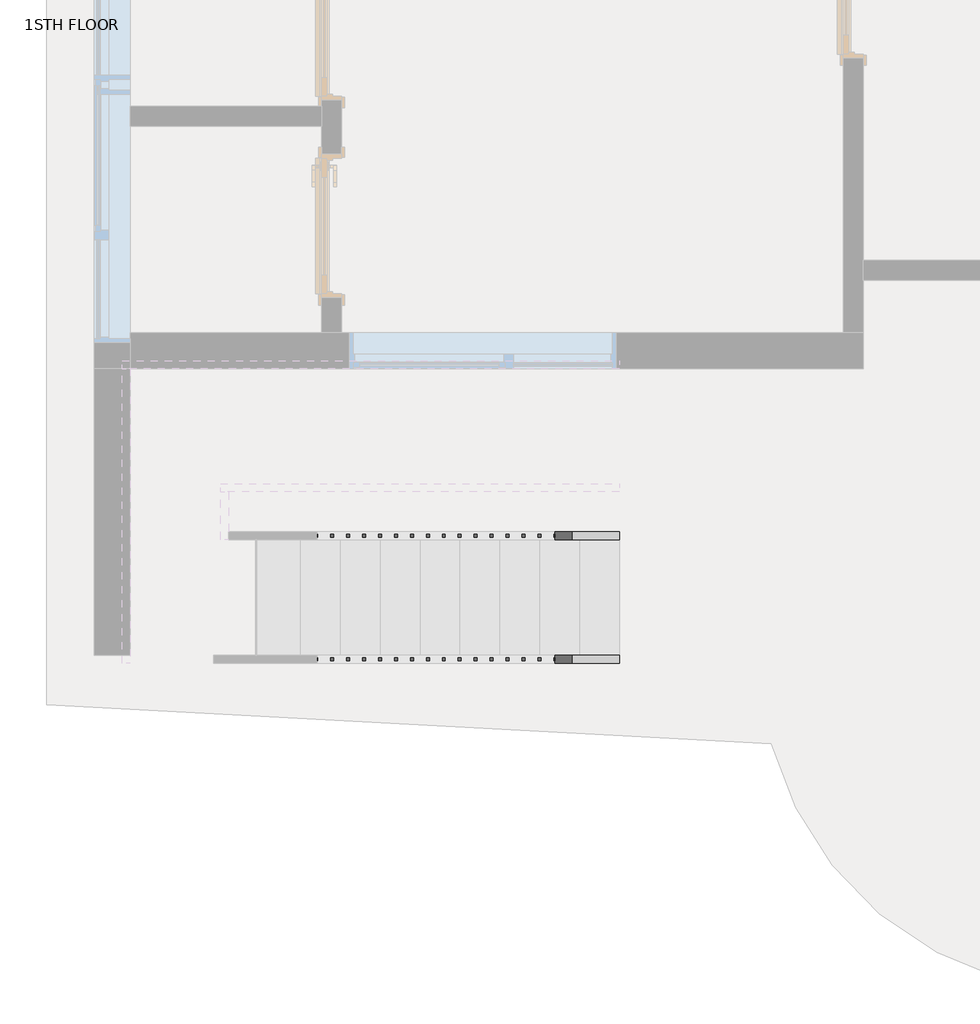
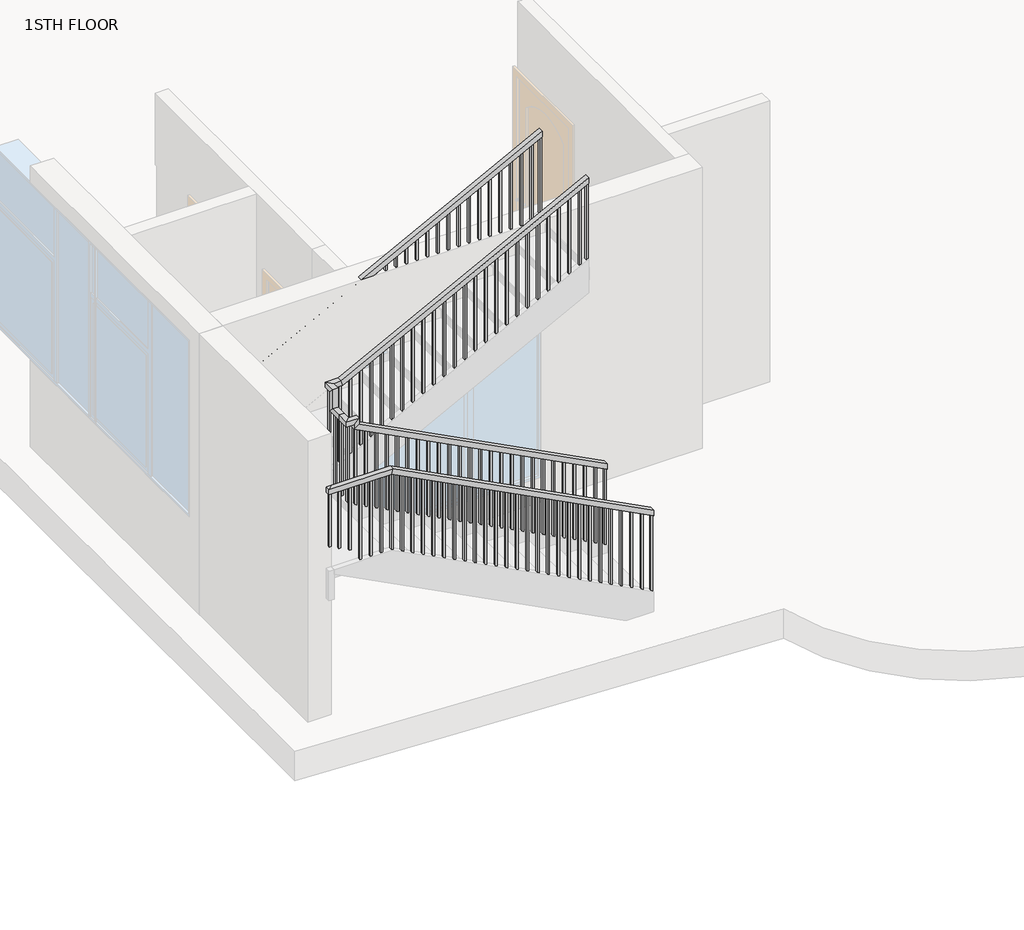
# One storey, part 3 of 4: 2 railings.
"""IFC4 building model written with IfcOpenShell, lengths in millimetres."""

from ifc_helpers import new_model, si_unit, frame, origin, place, context, project, spatial, polyline, outline, extrude, faceted_brep, element, save

model = new_model("IFC4")

# Units and contexts
model_context = context("Model", 3, world=origin())
ifc_project = project(units=[si_unit("LENGTHUNIT", "METRE", prefix="MILLI")], contexts=[model_context])

# Site, building, storey
site = spatial("IfcSite", under=ifc_project)
building = spatial("IfcBuilding", under=site)
storey = spatial("IfcBuildingStorey", under=building, Name="1STH FLOOR", Elevation=3200.4)

# Railings
placement = place(None, origin())
element("IfcRailing", 1, ObjectType="Handrail - Rectangular", at=placement, inside=storey, context=model_context, shape_type="SolidModel", body=[
    faceted_brep([(-3117.2664982, -6914.3822004, 4246.4181818), (-3117.2664982, -6914.3822004, 4189.203028), (-3117.2664982, -6863.5822004, 4189.203028), (-3117.2664982, -6863.5822004, 4246.4181818), (-5530.2664982, -6914.3822004, 5496.7909091), (-5581.0664982, -6914.3822004, 5465.8993916), (-5581.0664982, -6863.5822004, 5465.8993916), (-5530.2664982, -6863.5822004, 5496.7909091), (-5657.2664982, -6787.3822004, 5511.8), (-5657.2664982, -6787.3822004, 5562.6), (-5657.2664982, -6685.7822004, 5562.6), (-5657.2664982, -6634.9822004, 5511.8), (-5606.4664982, -6787.3822004, 5511.8), (-5606.4664982, -6634.9822004, 5511.8), (-5606.4664982, -6787.3822004, 5562.6), (-5606.4664982, -6685.7822004, 5562.6), (-3117.2664982, -6558.7822004, 7010.4), (-3117.2664982, -6609.5822004, 7010.4), (-3117.2664982, -6609.5822004, 6953.1848461), (-3117.2664982, -6558.7822004, 6953.1848461), (-5517.8863767, -6558.7822004, 5709.2272727), (-5530.2664982, -6558.7822004, 5760.0272727), (-5517.8863767, -6609.5822004, 5709.2272727), (-5530.2664982, -6609.5822004, 5760.0272727), (-5530.2664982, -6914.3822004, 5562.6), (-5581.0664982, -6914.3822004, 5511.8), (-5581.0664982, -6863.5822004, 5511.8), (-5530.2664982, -6863.5822004, 5562.6), (-5657.2664982, -6914.3822004, 5562.6), (-5657.2664982, -6914.3822004, 5511.8), (-5606.4664982, -6863.5822004, 5511.8), (-5606.4664982, -6863.5822004, 5562.6), (-5657.2664982, -6685.7822004, 5760.0272727), (-5657.2664982, -6634.9822004, 5709.2272727), (-5606.4664982, -6634.9822004, 5709.2272727), (-5606.4664982, -6685.7822004, 5760.0272727), (-5657.2664982, -6558.7822004, 5760.0272727), (-5657.2664982, -6558.7822004, 5709.2272727), (-5606.4664982, -6609.5822004, 5709.2272727), (-5606.4664982, -6609.5822004, 5760.0272727)], [[[0, 1, 2, 3]], [[1, 0, 4, 5]], [[2, 1, 5, 6]], [[3, 2, 6, 7]], [[0, 3, 7, 4]], [[8, 9, 10, 11]], [[12, 8, 11, 13]], [[14, 12, 13, 15]], [[9, 14, 15, 10]], [[16, 17, 18, 19]], [[20, 21, 16, 19]], [[22, 20, 19, 18]], [[23, 22, 18, 17]], [[21, 23, 17, 16]], [[5, 4, 24, 25]], [[6, 5, 25, 26]], [[7, 6, 26, 27]], [[4, 7, 27, 24]], [[25, 24, 28, 29]], [[26, 25, 29, 30]], [[27, 26, 30, 31]], [[24, 27, 31, 28]], [[29, 28, 9, 8]], [[30, 29, 8, 12]], [[31, 30, 12, 14]], [[28, 31, 14, 9]], [[11, 10, 32, 33]], [[13, 11, 33, 34]], [[15, 13, 34, 35]], [[10, 15, 35, 32]], [[33, 32, 36, 37]], [[34, 33, 37, 38]], [[35, 34, 38, 39]], [[32, 35, 39, 36]], [[37, 36, 21, 20]], [[38, 37, 20, 22]], [[39, 38, 22, 23]], [[36, 39, 23, 21]]]),
    extrude(outline(polyline([(6918.6350734, -3183.9414982), (6908.7637098, -3202.9914982), (6124.4803899, -3202.9914982), (6134.3517536, -3183.9414982), (6918.6350734, -3183.9414982)])), frame((0.0, -6593.7072004, 0.0), z_axis=(0.0, 1.0, 0.0), x_axis=(0.0, 0.0, 1.0)), (0.0, 0.0, 1.0), 19.05),
    extrude(outline(polyline([(6865.9878007, -3285.5414982), (6856.116437, -3304.5914982), (6071.8331172, -3304.5914982), (6081.7044808, -3285.5414982), (6865.9878007, -3285.5414982)])), frame((0.0, -6593.7072004, 0.0), z_axis=(0.0, 1.0, 0.0), x_axis=(0.0, 0.0, 1.0)), (0.0, 0.0, 1.0), 19.05),
    extrude(outline(polyline([(6813.340528, -3387.1414982), (6803.4691643, -3406.1914982), (6019.1858445, -3406.1914982), (6029.0572081, -3387.1414982), (6813.340528, -3387.1414982)])), frame((0.0, -6593.7072004, 0.0), z_axis=(0.0, 1.0, 0.0), x_axis=(0.0, 0.0, 1.0)), (0.0, 0.0, 1.0), 19.05),
    extrude(outline(polyline([(6760.6932552, -3488.7414982), (6750.8218916, -3507.7914982), (5966.5385718, -3507.7914982), (5976.4099354, -3488.7414982), (6760.6932552, -3488.7414982)])), frame((0.0, -6593.7072004, 0.0), z_axis=(0.0, 1.0, 0.0), x_axis=(0.0, 0.0, 1.0)), (0.0, 0.0, 1.0), 19.05),
    extrude(outline(polyline([(6708.0459825, -3590.3414982), (6698.1746189, -3609.3914982), (5913.891299, -3609.3914982), (5923.7626627, -3590.3414982), (6708.0459825, -3590.3414982)])), frame((0.0, -6593.7072004, 0.0), z_axis=(0.0, 1.0, 0.0), x_axis=(0.0, 0.0, 1.0)), (0.0, 0.0, 1.0), 19.05),
    extrude(outline(polyline([(6655.3987098, -3691.9414982), (6645.5273461, -3710.9914982), (5861.2440263, -3710.9914982), (5871.1153899, -3691.9414982), (6655.3987098, -3691.9414982)])), frame((0.0, -6593.7072004, 0.0), z_axis=(0.0, 1.0, 0.0), x_axis=(0.0, 0.0, 1.0)), (0.0, 0.0, 1.0), 19.05),
    extrude(outline(polyline([(6602.751437, -3793.5414982), (6592.8800734, -3812.5914982), (5808.5967536, -3812.5914982), (5818.4681172, -3793.5414982), (6602.751437, -3793.5414982)])), frame((0.0, -6593.7072004, 0.0), z_axis=(0.0, 1.0, 0.0), x_axis=(0.0, 0.0, 1.0)), (0.0, 0.0, 1.0), 19.05),
    extrude(outline(polyline([(6550.1041643, -3895.1414982), (6540.2328007, -3914.1914982), (5755.9494808, -3914.1914982), (5765.8208445, -3895.1414982), (6550.1041643, -3895.1414982)])), frame((0.0, -6593.7072004, 0.0), z_axis=(0.0, 1.0, 0.0), x_axis=(0.0, 0.0, 1.0)), (0.0, 0.0, 1.0), 19.05),
    extrude(outline(polyline([(6497.4568916, -3996.7414982), (6487.585528, -4015.7914982), (5703.3022081, -4015.7914982), (5713.1735718, -3996.7414982), (6497.4568916, -3996.7414982)])), frame((0.0, -6593.7072004, 0.0), z_axis=(0.0, 1.0, 0.0), x_axis=(0.0, 0.0, 1.0)), (0.0, 0.0, 1.0), 19.05),
    extrude(outline(polyline([(6444.8096189, -4098.3414982), (6434.9382552, -4117.3914982), (5650.6549354, -4117.3914982), (5660.526299, -4098.3414982), (6444.8096189, -4098.3414982)])), frame((0.0, -6593.7072004, 0.0), z_axis=(0.0, 1.0, 0.0), x_axis=(0.0, 0.0, 1.0)), (0.0, 0.0, 1.0), 19.05),
    extrude(outline(polyline([(6392.1623461, -4199.9414982), (6382.2909825, -4218.9914982), (5598.0076627, -4218.9914982), (5607.8790263, -4199.9414982), (6392.1623461, -4199.9414982)])), frame((0.0, -6593.7072004, 0.0), z_axis=(0.0, 1.0, 0.0), x_axis=(0.0, 0.0, 1.0)), (0.0, 0.0, 1.0), 19.05),
    extrude(outline(polyline([(6339.5150734, -4301.5414982), (6329.6437098, -4320.5914982), (5545.3603899, -4320.5914982), (5555.2317536, -4301.5414982), (6339.5150734, -4301.5414982)])), frame((0.0, -6593.7072004, 0.0), z_axis=(0.0, 1.0, 0.0), x_axis=(0.0, 0.0, 1.0)), (0.0, 0.0, 1.0), 19.05),
    extrude(outline(polyline([(6286.8678007, -4403.1414982), (6276.996437, -4422.1914982), (5492.7131172, -4422.1914982), (5502.5844808, -4403.1414982), (6286.8678007, -4403.1414982)])), frame((0.0, -6593.7072004, 0.0), z_axis=(0.0, 1.0, 0.0), x_axis=(0.0, 0.0, 1.0)), (0.0, 0.0, 1.0), 19.05),
    extrude(outline(polyline([(6234.220528, -4504.7414982), (6224.3491643, -4523.7914982), (5440.0658445, -4523.7914982), (5449.9372081, -4504.7414982), (6234.220528, -4504.7414982)])), frame((0.0, -6593.7072004, 0.0), z_axis=(0.0, 1.0, 0.0), x_axis=(0.0, 0.0, 1.0)), (0.0, 0.0, 1.0), 19.05),
    extrude(outline(polyline([(6181.5732552, -4606.3414982), (6171.7018916, -4625.3914982), (5387.4185718, -4625.3914982), (5397.2899354, -4606.3414982), (6181.5732552, -4606.3414982)])), frame((0.0, -6593.7072004, 0.0), z_axis=(0.0, 1.0, 0.0), x_axis=(0.0, 0.0, 1.0)), (0.0, 0.0, 1.0), 19.05),
    extrude(outline(polyline([(6128.9259825, -4707.9414982), (6119.0546189, -4726.9914982), (5334.771299, -4726.9914982), (5344.6426627, -4707.9414982), (6128.9259825, -4707.9414982)])), frame((0.0, -6593.7072004, 0.0), z_axis=(0.0, 1.0, 0.0), x_axis=(0.0, 0.0, 1.0)), (0.0, 0.0, 1.0), 19.05),
    extrude(outline(polyline([(6076.2787098, -4809.5414982), (6066.4073461, -4828.5914982), (5282.1240263, -4828.5914982), (5291.9953899, -4809.5414982), (6076.2787098, -4809.5414982)])), frame((0.0, -6593.7072004, 0.0), z_axis=(0.0, 1.0, 0.0), x_axis=(0.0, 0.0, 1.0)), (0.0, 0.0, 1.0), 19.05),
    extrude(outline(polyline([(6023.631437, -4911.1414982), (6013.7600734, -4930.1914982), (5229.4767536, -4930.1914982), (5239.3481172, -4911.1414982), (6023.631437, -4911.1414982)])), frame((0.0, -6593.7072004, 0.0), z_axis=(0.0, 1.0, 0.0), x_axis=(0.0, 0.0, 1.0)), (0.0, 0.0, 1.0), 19.05),
    extrude(outline(polyline([(5970.9841643, -5012.7414982), (5961.1128007, -5031.7914982), (5176.8294808, -5031.7914982), (5186.7008445, -5012.7414982), (5970.9841643, -5012.7414982)])), frame((0.0, -6593.7072004, 0.0), z_axis=(0.0, 1.0, 0.0), x_axis=(0.0, 0.0, 1.0)), (0.0, 0.0, 1.0), 19.05),
    extrude(outline(polyline([(5918.3368916, -5114.3414982), (5908.465528, -5133.3914982), (5124.1822081, -5133.3914982), (5134.0535718, -5114.3414982), (5918.3368916, -5114.3414982)])), frame((0.0, -6593.7072004, 0.0), z_axis=(0.0, 1.0, 0.0), x_axis=(0.0, 0.0, 1.0)), (0.0, 0.0, 1.0), 19.05),
    extrude(outline(polyline([(5865.6896189, -5215.9414982), (5855.8182552, -5234.9914982), (5071.5349354, -5234.9914982), (5081.406299, -5215.9414982), (5865.6896189, -5215.9414982)])), frame((0.0, -6593.7072004, 0.0), z_axis=(0.0, 1.0, 0.0), x_axis=(0.0, 0.0, 1.0)), (0.0, 0.0, 1.0), 19.05),
    extrude(outline(polyline([(5813.0423461, -5317.5414982), (5803.1709825, -5336.5914982), (5018.8876627, -5336.5914982), (5028.7590263, -5317.5414982), (5813.0423461, -5317.5414982)])), frame((0.0, -6593.7072004, 0.0), z_axis=(0.0, 1.0, 0.0), x_axis=(0.0, 0.0, 1.0)), (0.0, 0.0, 1.0), 19.05),
    extrude(outline(polyline([(5760.3950734, -5419.1414982), (5750.5237098, -5438.1914982), (4966.2403899, -5438.1914982), (4976.1117536, -5419.1414982), (5760.3950734, -5419.1414982)])), frame((0.0, -6593.7072004, 0.0), z_axis=(0.0, 1.0, 0.0), x_axis=(0.0, 0.0, 1.0)), (0.0, 0.0, 1.0), 19.05),
    extrude(outline(polyline([(5707.7478007, -5520.7414982), (5697.876437, -5539.7914982), (4913.5931172, -5539.7914982), (4923.4644808, -5520.7414982), (5707.7478007, -5520.7414982)])), frame((0.0, -6593.7072004, 0.0), z_axis=(0.0, 1.0, 0.0), x_axis=(0.0, 0.0, 1.0)), (0.0, 0.0, 1.0), 19.05),
    extrude(outline(polyline([(-5622.3414982, -6695.3072004), (-5641.3914982, -6695.3072004), (-5641.3914982, -6676.2572004), (-5622.3414982, -6676.2572004), (-5622.3414982, -6695.3072004)])), frame((0.0, 0.0, 4724.4), z_axis=(0.0, 0.0, 1.0), x_axis=(1.0, 0.0, 0.0)), (0.0, 0.0, 1.0), 787.4),
    extrude(outline(polyline([(-5622.3414982, -6796.9072004), (-5641.3914982, -6796.9072004), (-5641.3914982, -6777.8572004), (-5622.3414982, -6777.8572004), (-5622.3414982, -6796.9072004)])), frame((0.0, 0.0, 4724.4), z_axis=(0.0, 0.0, 1.0), x_axis=(1.0, 0.0, 0.0)), (0.0, 0.0, 1.0), 787.4),
    extrude(outline(polyline([(5511.8, -5546.1414982), (5511.8, -5565.1914982), (4673.3899354, -5565.1914982), (4663.5185718, -5546.1414982), (5511.8, -5546.1414982)])), frame((0.0, -6898.5072004, 0.0), z_axis=(0.0, 1.0, 0.0), x_axis=(0.0, 0.0, 1.0)), (0.0, 0.0, 1.0), 19.05),
    extrude(outline(polyline([(5395.1546189, -5444.5414982), (5405.0259825, -5463.5914982), (4620.7426627, -5463.5914982), (4610.871299, -5444.5414982), (5395.1546189, -5444.5414982)])), frame((0.0, -6898.5072004, 0.0), z_axis=(0.0, 1.0, 0.0), x_axis=(0.0, 0.0, 1.0)), (0.0, 0.0, 1.0), 19.05),
    extrude(outline(polyline([(5342.5073461, -5342.9414982), (5352.3787098, -5361.9914982), (4568.0953899, -5361.9914982), (4558.2240263, -5342.9414982), (5342.5073461, -5342.9414982)])), frame((0.0, -6898.5072004, 0.0), z_axis=(0.0, 1.0, 0.0), x_axis=(0.0, 0.0, 1.0)), (0.0, 0.0, 1.0), 19.05),
    extrude(outline(polyline([(5289.8600734, -5241.3414982), (5299.731437, -5260.3914982), (4515.4481172, -5260.3914982), (4505.5767536, -5241.3414982), (5289.8600734, -5241.3414982)])), frame((0.0, -6898.5072004, 0.0), z_axis=(0.0, 1.0, 0.0), x_axis=(0.0, 0.0, 1.0)), (0.0, 0.0, 1.0), 19.05),
    extrude(outline(polyline([(5237.2128007, -5139.7414982), (5247.0841643, -5158.7914982), (4462.8008445, -5158.7914982), (4452.9294808, -5139.7414982), (5237.2128007, -5139.7414982)])), frame((0.0, -6898.5072004, 0.0), z_axis=(0.0, 1.0, 0.0), x_axis=(0.0, 0.0, 1.0)), (0.0, 0.0, 1.0), 19.05),
    extrude(outline(polyline([(5184.565528, -5038.1414982), (5194.4368916, -5057.1914982), (4410.1535718, -5057.1914982), (4400.2822081, -5038.1414982), (5184.565528, -5038.1414982)])), frame((0.0, -6898.5072004, 0.0), z_axis=(0.0, 1.0, 0.0), x_axis=(0.0, 0.0, 1.0)), (0.0, 0.0, 1.0), 19.05),
    extrude(outline(polyline([(5131.9182552, -4936.5414982), (5141.7896189, -4955.5914982), (4357.506299, -4955.5914982), (4347.6349354, -4936.5414982), (5131.9182552, -4936.5414982)])), frame((0.0, -6898.5072004, 0.0), z_axis=(0.0, 1.0, 0.0), x_axis=(0.0, 0.0, 1.0)), (0.0, 0.0, 1.0), 19.05),
    extrude(outline(polyline([(5079.2709825, -4834.9414982), (5089.1423461, -4853.9914982), (4304.8590263, -4853.9914982), (4294.9876627, -4834.9414982), (5079.2709825, -4834.9414982)])), frame((0.0, -6898.5072004, 0.0), z_axis=(0.0, 1.0, 0.0), x_axis=(0.0, 0.0, 1.0)), (0.0, 0.0, 1.0), 19.05),
    extrude(outline(polyline([(5026.6237098, -4733.3414982), (5036.4950734, -4752.3914982), (4252.2117536, -4752.3914982), (4242.3403899, -4733.3414982), (5026.6237098, -4733.3414982)])), frame((0.0, -6898.5072004, 0.0), z_axis=(0.0, 1.0, 0.0), x_axis=(0.0, 0.0, 1.0)), (0.0, 0.0, 1.0), 19.05),
    extrude(outline(polyline([(4973.976437, -4631.7414982), (4983.8478007, -4650.7914982), (4199.5644808, -4650.7914982), (4189.6931172, -4631.7414982), (4973.976437, -4631.7414982)])), frame((0.0, -6898.5072004, 0.0), z_axis=(0.0, 1.0, 0.0), x_axis=(0.0, 0.0, 1.0)), (0.0, 0.0, 1.0), 19.05),
    extrude(outline(polyline([(4921.3291643, -4530.1414982), (4931.200528, -4549.1914982), (4146.9172081, -4549.1914982), (4137.0458445, -4530.1414982), (4921.3291643, -4530.1414982)])), frame((0.0, -6898.5072004, 0.0), z_axis=(0.0, 1.0, 0.0), x_axis=(0.0, 0.0, 1.0)), (0.0, 0.0, 1.0), 19.05),
    extrude(outline(polyline([(4868.6818916, -4428.5414982), (4878.5532552, -4447.5914982), (4094.2699354, -4447.5914982), (4084.3985718, -4428.5414982), (4868.6818916, -4428.5414982)])), frame((0.0, -6898.5072004, 0.0), z_axis=(0.0, 1.0, 0.0), x_axis=(0.0, 0.0, 1.0)), (0.0, 0.0, 1.0), 19.05),
    extrude(outline(polyline([(4816.0346189, -4326.9414982), (4825.9059825, -4345.9914982), (4041.6226627, -4345.9914982), (4031.751299, -4326.9414982), (4816.0346189, -4326.9414982)])), frame((0.0, -6898.5072004, 0.0), z_axis=(0.0, 1.0, 0.0), x_axis=(0.0, 0.0, 1.0)), (0.0, 0.0, 1.0), 19.05),
    extrude(outline(polyline([(4763.3873461, -4225.3414982), (4773.2587098, -4244.3914982), (3988.9753899, -4244.3914982), (3979.1040263, -4225.3414982), (4763.3873461, -4225.3414982)])), frame((0.0, -6898.5072004, 0.0), z_axis=(0.0, 1.0, 0.0), x_axis=(0.0, 0.0, 1.0)), (0.0, 0.0, 1.0), 19.05),
    extrude(outline(polyline([(4710.7400734, -4123.7414982), (4720.611437, -4142.7914982), (3936.3281172, -4142.7914982), (3926.4567536, -4123.7414982), (4710.7400734, -4123.7414982)])), frame((0.0, -6898.5072004, 0.0), z_axis=(0.0, 1.0, 0.0), x_axis=(0.0, 0.0, 1.0)), (0.0, 0.0, 1.0), 19.05),
    extrude(outline(polyline([(4658.0928007, -4022.1414982), (4667.9641643, -4041.1914982), (3883.6808445, -4041.1914982), (3873.8094808, -4022.1414982), (4658.0928007, -4022.1414982)])), frame((0.0, -6898.5072004, 0.0), z_axis=(0.0, 1.0, 0.0), x_axis=(0.0, 0.0, 1.0)), (0.0, 0.0, 1.0), 19.05),
    extrude(outline(polyline([(4605.445528, -3920.5414982), (4615.3168916, -3939.5914982), (3831.0335718, -3939.5914982), (3821.1622081, -3920.5414982), (4605.445528, -3920.5414982)])), frame((0.0, -6898.5072004, 0.0), z_axis=(0.0, 1.0, 0.0), x_axis=(0.0, 0.0, 1.0)), (0.0, 0.0, 1.0), 19.05),
    extrude(outline(polyline([(4552.7982552, -3818.9414982), (4562.6696189, -3837.9914982), (3778.386299, -3837.9914982), (3768.5149354, -3818.9414982), (4552.7982552, -3818.9414982)])), frame((0.0, -6898.5072004, 0.0), z_axis=(0.0, 1.0, 0.0), x_axis=(0.0, 0.0, 1.0)), (0.0, 0.0, 1.0), 19.05),
    extrude(outline(polyline([(4500.1509825, -3717.3414982), (4510.0223461, -3736.3914982), (3725.7390263, -3736.3914982), (3715.8676627, -3717.3414982), (4500.1509825, -3717.3414982)])), frame((0.0, -6898.5072004, 0.0), z_axis=(0.0, 1.0, 0.0), x_axis=(0.0, 0.0, 1.0)), (0.0, 0.0, 1.0), 19.05),
    extrude(outline(polyline([(4447.5037098, -3615.7414982), (4457.3750734, -3634.7914982), (3673.0917536, -3634.7914982), (3663.2203899, -3615.7414982), (4447.5037098, -3615.7414982)])), frame((0.0, -6898.5072004, 0.0), z_axis=(0.0, 1.0, 0.0), x_axis=(0.0, 0.0, 1.0)), (0.0, 0.0, 1.0), 19.05),
    extrude(outline(polyline([(4394.856437, -3514.1414982), (4404.7278007, -3533.1914982), (3620.4444808, -3533.1914982), (3610.5731172, -3514.1414982), (4394.856437, -3514.1414982)])), frame((0.0, -6898.5072004, 0.0), z_axis=(0.0, 1.0, 0.0), x_axis=(0.0, 0.0, 1.0)), (0.0, 0.0, 1.0), 19.05),
    extrude(outline(polyline([(4342.2091643, -3412.5414982), (4352.080528, -3431.5914982), (3567.7972081, -3431.5914982), (3557.9258445, -3412.5414982), (4342.2091643, -3412.5414982)])), frame((0.0, -6898.5072004, 0.0), z_axis=(0.0, 1.0, 0.0), x_axis=(0.0, 0.0, 1.0)), (0.0, 0.0, 1.0), 19.05),
    extrude(outline(polyline([(4289.5618916, -3310.9414982), (4299.4332552, -3329.9914982), (3515.1499354, -3329.9914982), (3505.2785718, -3310.9414982), (4289.5618916, -3310.9414982)])), frame((0.0, -6898.5072004, 0.0), z_axis=(0.0, 1.0, 0.0), x_axis=(0.0, 0.0, 1.0)), (0.0, 0.0, 1.0), 19.05),
    extrude(outline(polyline([(4236.9146189, -3209.3414982), (4246.7859825, -3228.3914982), (3462.5026627, -3228.3914982), (3452.631299, -3209.3414982), (4236.9146189, -3209.3414982)])), frame((0.0, -6898.5072004, 0.0), z_axis=(0.0, 1.0, 0.0), x_axis=(0.0, 0.0, 1.0)), (0.0, 0.0, 1.0), 19.05),
    extrude(outline(polyline([(-6593.7072004, 5709.2272727), (-6574.6572004, 5709.2272727), (-6574.6572004, 4870.8172081), (-6593.7072004, 4860.9458445), (-6593.7072004, 5709.2272727)])), frame((-5641.3914982, 0.0, 0.0), z_axis=(1.0, 0.0, 0.0), x_axis=(0.0, 1.0, 0.0)), (0.0, 0.0, 1.0), 19.05),
    extrude(outline(polyline([(-5622.3414982, -6879.4572004), (-5622.3414982, -6898.5072004), (-5641.3914982, -6898.5072004), (-5641.3914982, -6879.4572004), (-5622.3414982, -6879.4572004)])), frame((0.0, 0.0, 4724.4), z_axis=(0.0, 0.0, 1.0), x_axis=(1.0, 0.0, 0.0)), (0.0, 0.0, 1.0), 787.4),
    extrude(outline(polyline([(6953.1848461, -3117.2664982), (6943.3134825, -3136.3164982), (6159.0301627, -3136.3164982), (6168.9015263, -3117.2664982), (6953.1848461, -3117.2664982)])), frame((0.0, -6593.7072004, 0.0), z_axis=(0.0, 1.0, 0.0), x_axis=(0.0, 0.0, 1.0)), (0.0, 0.0, 1.0), 19.05),
    extrude(outline(polyline([(4189.203028, -3117.2664982), (4199.0743916, -3136.3164982), (3414.7910718, -3136.3164982), (3404.9197081, -3117.2664982), (4189.203028, -3117.2664982)])), frame((0.0, -6898.5072004, 0.0), z_axis=(0.0, 1.0, 0.0), x_axis=(0.0, 0.0, 1.0)), (0.0, 0.0, 1.0), 19.05),
])
element("IfcRailing", 2, ObjectType="Handrail - Rectangular", at=placement, inside=storey, context=model_context, shape_type="SolidModel", body=[
    faceted_brep([(-3117.2664982, -7701.7822004, 4246.4181818), (-3117.2664982, -7701.7822004, 4189.203028), (-3117.2664982, -7650.9822004, 4189.203028), (-3117.2664982, -7650.9822004, 4246.4181818), (-5657.2664982, -7701.7822004, 5562.6), (-5669.6466197, -7701.7822004, 5511.8), (-5669.6466197, -7650.9822004, 5511.8), (-5657.2664982, -7650.9822004, 5562.6), (-6283.3131972, -7701.7822004, 5511.8), (-6283.3131972, -7701.7822004, 5562.6), (-6283.3131972, -5773.9082131, 5562.6), (-6283.3131972, -5773.9082131, 5511.8), (-6232.5131972, -7650.9822004, 5511.8), (-6232.5131972, -5824.7082131, 5511.8), (-6232.5131972, -7650.9822004, 5562.6), (-6232.5131972, -5824.7082131, 5562.6), (-5911.2664982, -5773.9082131, 5562.6), (-5898.8863767, -5773.9082131, 5511.8), (-5898.8863767, -5824.7082131, 5511.8), (-5911.2664982, -5824.7082131, 5562.6), (-3117.2664982, -5773.9082131, 7010.4), (-3117.2664982, -5824.7082131, 7010.4), (-3117.2664982, -5824.7082131, 6953.1848461), (-3117.2664982, -5773.9082131, 6953.1848461)], [[[0, 1, 2, 3]], [[1, 0, 4, 5]], [[2, 1, 5, 6]], [[3, 2, 6, 7]], [[0, 3, 7, 4]], [[8, 9, 10, 11]], [[12, 8, 11, 13]], [[14, 12, 13, 15]], [[9, 14, 15, 10]], [[11, 10, 16, 17]], [[13, 11, 17, 18]], [[15, 13, 18, 19]], [[10, 15, 19, 16]], [[5, 4, 9, 8]], [[6, 5, 8, 12]], [[7, 6, 12, 14]], [[4, 7, 14, 9]], [[20, 21, 22, 23]], [[17, 16, 20, 23]], [[18, 17, 23, 22]], [[19, 18, 22, 21]], [[16, 19, 21, 20]]]),
    extrude(outline(polyline([(6900.2413294, -3219.4381972), (6115.9580095, -3219.4381972), (6125.8293732, -3200.3881972), (6910.112693, -3200.3881972), (6900.2413294, -3219.4381972)])), frame((0.0, -5808.8332131, 0.0), z_axis=(0.0, 1.0, 0.0), x_axis=(0.0, 0.0, 1.0)), (0.0, 0.0, 1.0), 19.05),
    extrude(outline(polyline([(6847.5940566, -3321.0381972), (6063.3107368, -3321.0381972), (6073.1821004, -3301.9881972), (6857.4654203, -3301.9881972), (6847.5940566, -3321.0381972)])), frame((0.0, -5808.8332131, 0.0), z_axis=(0.0, 1.0, 0.0), x_axis=(0.0, 0.0, 1.0)), (0.0, 0.0, 1.0), 19.05),
    extrude(outline(polyline([(6794.9467839, -3422.6381972), (6010.6634641, -3422.6381972), (6020.5348277, -3403.5881972), (6804.8181476, -3403.5881972), (6794.9467839, -3422.6381972)])), frame((0.0, -5808.8332131, 0.0), z_axis=(0.0, 1.0, 0.0), x_axis=(0.0, 0.0, 1.0)), (0.0, 0.0, 1.0), 19.05),
    extrude(outline(polyline([(6742.2995112, -3524.2381972), (5958.0161913, -3524.2381972), (5967.887555, -3505.1881972), (6752.1708748, -3505.1881972), (6742.2995112, -3524.2381972)])), frame((0.0, -5808.8332131, 0.0), z_axis=(0.0, 1.0, 0.0), x_axis=(0.0, 0.0, 1.0)), (0.0, 0.0, 1.0), 19.05),
    extrude(outline(polyline([(6689.6522385, -3625.8381972), (5905.3689186, -3625.8381972), (5915.2402823, -3606.7881972), (6699.5236021, -3606.7881972), (6689.6522385, -3625.8381972)])), frame((0.0, -5808.8332131, 0.0), z_axis=(0.0, 1.0, 0.0), x_axis=(0.0, 0.0, 1.0)), (0.0, 0.0, 1.0), 19.05),
    extrude(outline(polyline([(6637.0049657, -3727.4381972), (5852.7216459, -3727.4381972), (5862.5930095, -3708.3881972), (6646.8763294, -3708.3881972), (6637.0049657, -3727.4381972)])), frame((0.0, -5808.8332131, 0.0), z_axis=(0.0, 1.0, 0.0), x_axis=(0.0, 0.0, 1.0)), (0.0, 0.0, 1.0), 19.05),
    extrude(outline(polyline([(6584.357693, -3829.0381972), (5800.0743732, -3829.0381972), (5809.9457368, -3809.9881972), (6594.2290566, -3809.9881972), (6584.357693, -3829.0381972)])), frame((0.0, -5808.8332131, 0.0), z_axis=(0.0, 1.0, 0.0), x_axis=(0.0, 0.0, 1.0)), (0.0, 0.0, 1.0), 19.05),
    extrude(outline(polyline([(6531.7104203, -3930.6381972), (5747.4271004, -3930.6381972), (5757.2984641, -3911.5881972), (6541.5817839, -3911.5881972), (6531.7104203, -3930.6381972)])), frame((0.0, -5808.8332131, 0.0), z_axis=(0.0, 1.0, 0.0), x_axis=(0.0, 0.0, 1.0)), (0.0, 0.0, 1.0), 19.05),
    extrude(outline(polyline([(6479.0631476, -4032.2381972), (5694.7798277, -4032.2381972), (5704.6511913, -4013.1881972), (6488.9345112, -4013.1881972), (6479.0631476, -4032.2381972)])), frame((0.0, -5808.8332131, 0.0), z_axis=(0.0, 1.0, 0.0), x_axis=(0.0, 0.0, 1.0)), (0.0, 0.0, 1.0), 19.05),
    extrude(outline(polyline([(6426.4158748, -4133.8381972), (5642.132555, -4133.8381972), (5652.0039186, -4114.7881972), (6436.2872385, -4114.7881972), (6426.4158748, -4133.8381972)])), frame((0.0, -5808.8332131, 0.0), z_axis=(0.0, 1.0, 0.0), x_axis=(0.0, 0.0, 1.0)), (0.0, 0.0, 1.0), 19.05),
    extrude(outline(polyline([(6373.7686021, -4235.4381972), (5589.4852823, -4235.4381972), (5599.3566459, -4216.3881972), (6383.6399657, -4216.3881972), (6373.7686021, -4235.4381972)])), frame((0.0, -5808.8332131, 0.0), z_axis=(0.0, 1.0, 0.0), x_axis=(0.0, 0.0, 1.0)), (0.0, 0.0, 1.0), 19.05),
    extrude(outline(polyline([(6321.1213294, -4337.0381972), (5536.8380095, -4337.0381972), (5546.7093732, -4317.9881972), (6330.992693, -4317.9881972), (6321.1213294, -4337.0381972)])), frame((0.0, -5808.8332131, 0.0), z_axis=(0.0, 1.0, 0.0), x_axis=(0.0, 0.0, 1.0)), (0.0, 0.0, 1.0), 19.05),
    extrude(outline(polyline([(6268.4740566, -4438.6381972), (5484.1907368, -4438.6381972), (5494.0621004, -4419.5881972), (6278.3454203, -4419.5881972), (6268.4740566, -4438.6381972)])), frame((0.0, -5808.8332131, 0.0), z_axis=(0.0, 1.0, 0.0), x_axis=(0.0, 0.0, 1.0)), (0.0, 0.0, 1.0), 19.05),
    extrude(outline(polyline([(6215.8267839, -4540.2381972), (5431.5434641, -4540.2381972), (5441.4148277, -4521.1881972), (6225.6981476, -4521.1881972), (6215.8267839, -4540.2381972)])), frame((0.0, -5808.8332131, 0.0), z_axis=(0.0, 1.0, 0.0), x_axis=(0.0, 0.0, 1.0)), (0.0, 0.0, 1.0), 19.05),
    extrude(outline(polyline([(6163.1795112, -4641.8381972), (5378.8961913, -4641.8381972), (5388.767555, -4622.7881972), (6173.0508748, -4622.7881972), (6163.1795112, -4641.8381972)])), frame((0.0, -5808.8332131, 0.0), z_axis=(0.0, 1.0, 0.0), x_axis=(0.0, 0.0, 1.0)), (0.0, 0.0, 1.0), 19.05),
    extrude(outline(polyline([(6110.5322385, -4743.4381972), (5326.2489186, -4743.4381972), (5336.1202823, -4724.3881972), (6120.4036021, -4724.3881972), (6110.5322385, -4743.4381972)])), frame((0.0, -5808.8332131, 0.0), z_axis=(0.0, 1.0, 0.0), x_axis=(0.0, 0.0, 1.0)), (0.0, 0.0, 1.0), 19.05),
    extrude(outline(polyline([(6057.8849657, -4845.0381972), (5273.6016459, -4845.0381972), (5283.4730095, -4825.9881972), (6067.7563294, -4825.9881972), (6057.8849657, -4845.0381972)])), frame((0.0, -5808.8332131, 0.0), z_axis=(0.0, 1.0, 0.0), x_axis=(0.0, 0.0, 1.0)), (0.0, 0.0, 1.0), 19.05),
    extrude(outline(polyline([(6005.237693, -4946.6381972), (5220.9543732, -4946.6381972), (5230.8257368, -4927.5881972), (6015.1090566, -4927.5881972), (6005.237693, -4946.6381972)])), frame((0.0, -5808.8332131, 0.0), z_axis=(0.0, 1.0, 0.0), x_axis=(0.0, 0.0, 1.0)), (0.0, 0.0, 1.0), 19.05),
    extrude(outline(polyline([(5952.5904203, -5048.2381972), (5168.3071004, -5048.2381972), (5178.1784641, -5029.1881972), (5962.4617839, -5029.1881972), (5952.5904203, -5048.2381972)])), frame((0.0, -5808.8332131, 0.0), z_axis=(0.0, 1.0, 0.0), x_axis=(0.0, 0.0, 1.0)), (0.0, 0.0, 1.0), 19.05),
    extrude(outline(polyline([(5899.9431476, -5149.8381972), (5115.6598277, -5149.8381972), (5125.5311913, -5130.7881972), (5909.8145112, -5130.7881972), (5899.9431476, -5149.8381972)])), frame((0.0, -5808.8332131, 0.0), z_axis=(0.0, 1.0, 0.0), x_axis=(0.0, 0.0, 1.0)), (0.0, 0.0, 1.0), 19.05),
    extrude(outline(polyline([(5847.2958748, -5251.4381972), (5063.012555, -5251.4381972), (5072.8839186, -5232.3881972), (5857.1672385, -5232.3881972), (5847.2958748, -5251.4381972)])), frame((0.0, -5808.8332131, 0.0), z_axis=(0.0, 1.0, 0.0), x_axis=(0.0, 0.0, 1.0)), (0.0, 0.0, 1.0), 19.05),
    extrude(outline(polyline([(5794.6486021, -5353.0381972), (5010.3652823, -5353.0381972), (5020.2366459, -5333.9881972), (5804.5199657, -5333.9881972), (5794.6486021, -5353.0381972)])), frame((0.0, -5808.8332131, 0.0), z_axis=(0.0, 1.0, 0.0), x_axis=(0.0, 0.0, 1.0)), (0.0, 0.0, 1.0), 19.05),
    extrude(outline(polyline([(5742.0013294, -5454.6381972), (4957.7180095, -5454.6381972), (4967.5893732, -5435.5881972), (5751.872693, -5435.5881972), (5742.0013294, -5454.6381972)])), frame((0.0, -5808.8332131, 0.0), z_axis=(0.0, 1.0, 0.0), x_axis=(0.0, 0.0, 1.0)), (0.0, 0.0, 1.0), 19.05),
    extrude(outline(polyline([(5689.3540566, -5556.2381972), (4905.0707368, -5556.2381972), (4914.9421004, -5537.1881972), (5699.2254203, -5537.1881972), (5689.3540566, -5556.2381972)])), frame((0.0, -5808.8332131, 0.0), z_axis=(0.0, 1.0, 0.0), x_axis=(0.0, 0.0, 1.0)), (0.0, 0.0, 1.0), 19.05),
    extrude(outline(polyline([(5636.7067839, -5657.8381972), (4852.4234641, -5657.8381972), (4862.2948277, -5638.7881972), (5646.5781476, -5638.7881972), (5636.7067839, -5657.8381972)])), frame((0.0, -5808.8332131, 0.0), z_axis=(0.0, 1.0, 0.0), x_axis=(0.0, 0.0, 1.0)), (0.0, 0.0, 1.0), 19.05),
    extrude(outline(polyline([(5584.0595112, -5759.4381972), (4799.7761913, -5759.4381972), (4809.647555, -5740.3881972), (5593.9308748, -5740.3881972), (5584.0595112, -5759.4381972)])), frame((0.0, -5808.8332131, 0.0), z_axis=(0.0, 1.0, 0.0), x_axis=(0.0, 0.0, 1.0)), (0.0, 0.0, 1.0), 19.05),
    extrude(outline(polyline([(5531.4122385, -5861.0381972), (4747.1289186, -5861.0381972), (4757.0002823, -5841.9881972), (5541.2836021, -5841.9881972), (5531.4122385, -5861.0381972)])), frame((0.0, -5808.8332131, 0.0), z_axis=(0.0, 1.0, 0.0), x_axis=(0.0, 0.0, 1.0)), (0.0, 0.0, 1.0), 19.05),
    extrude(outline(polyline([(5511.8, -5962.6381972), (4694.4816459, -5962.6381972), (4704.3530095, -5943.5881972), (5511.8, -5943.5881972), (5511.8, -5962.6381972)])), frame((0.0, -5808.8332131, 0.0), z_axis=(0.0, 1.0, 0.0), x_axis=(0.0, 0.0, 1.0)), (0.0, 0.0, 1.0), 19.05),
    extrude(outline(polyline([(5511.8, -6064.2381972), (4641.8343732, -6064.2381972), (4651.7057368, -6045.1881972), (5511.8, -6045.1881972), (5511.8, -6064.2381972)])), frame((0.0, -5808.8332131, 0.0), z_axis=(0.0, 1.0, 0.0), x_axis=(0.0, 0.0, 1.0)), (0.0, 0.0, 1.0), 19.05),
    extrude(outline(polyline([(5511.8, -6165.8381972), (4589.1871004, -6165.8381972), (4599.0584641, -6146.7881972), (5511.8, -6146.7881972), (5511.8, -6165.8381972)])), frame((0.0, -5808.8332131, 0.0), z_axis=(0.0, 1.0, 0.0), x_axis=(0.0, 0.0, 1.0)), (0.0, 0.0, 1.0), 19.05),
    extrude(outline(polyline([(-6267.4381972, -5857.1072004), (-6267.4381972, -5838.0572004), (-6248.3881972, -5838.0572004), (-6248.3881972, -5857.1072004), (-6267.4381972, -5857.1072004)])), frame((0.0, 0.0, 4724.4), z_axis=(0.0, 0.0, 1.0), x_axis=(1.0, 0.0, 0.0)), (0.0, 0.0, 1.0), 787.4),
    extrude(outline(polyline([(-6267.4381972, -5958.7072004), (-6267.4381972, -5939.6572004), (-6248.3881972, -5939.6572004), (-6248.3881972, -5958.7072004), (-6267.4381972, -5958.7072004)])), frame((0.0, 0.0, 4724.4), z_axis=(0.0, 0.0, 1.0), x_axis=(1.0, 0.0, 0.0)), (0.0, 0.0, 1.0), 787.4),
    extrude(outline(polyline([(-6267.4381972, -6060.3072004), (-6267.4381972, -6041.2572004), (-6248.3881972, -6041.2572004), (-6248.3881972, -6060.3072004), (-6267.4381972, -6060.3072004)])), frame((0.0, 0.0, 4724.4), z_axis=(0.0, 0.0, 1.0), x_axis=(1.0, 0.0, 0.0)), (0.0, 0.0, 1.0), 787.4),
    extrude(outline(polyline([(-6267.4381972, -6161.9072004), (-6267.4381972, -6142.8572004), (-6248.3881972, -6142.8572004), (-6248.3881972, -6161.9072004), (-6267.4381972, -6161.9072004)])), frame((0.0, 0.0, 4724.4), z_axis=(0.0, 0.0, 1.0), x_axis=(1.0, 0.0, 0.0)), (0.0, 0.0, 1.0), 787.4),
    extrude(outline(polyline([(-6267.4381972, -6263.5072004), (-6267.4381972, -6244.4572004), (-6248.3881972, -6244.4572004), (-6248.3881972, -6263.5072004), (-6267.4381972, -6263.5072004)])), frame((0.0, 0.0, 4724.4), z_axis=(0.0, 0.0, 1.0), x_axis=(1.0, 0.0, 0.0)), (0.0, 0.0, 1.0), 787.4),
    extrude(outline(polyline([(-6267.4381972, -6365.1072004), (-6267.4381972, -6346.0572004), (-6248.3881972, -6346.0572004), (-6248.3881972, -6365.1072004), (-6267.4381972, -6365.1072004)])), frame((0.0, 0.0, 4724.4), z_axis=(0.0, 0.0, 1.0), x_axis=(1.0, 0.0, 0.0)), (0.0, 0.0, 1.0), 787.4),
    extrude(outline(polyline([(-6267.4381972, -6466.7072004), (-6267.4381972, -6447.6572004), (-6248.3881972, -6447.6572004), (-6248.3881972, -6466.7072004), (-6267.4381972, -6466.7072004)])), frame((0.0, 0.0, 4724.4), z_axis=(0.0, 0.0, 1.0), x_axis=(1.0, 0.0, 0.0)), (0.0, 0.0, 1.0), 787.4),
    extrude(outline(polyline([(-6267.4381972, -6568.3072004), (-6267.4381972, -6549.2572004), (-6248.3881972, -6549.2572004), (-6248.3881972, -6568.3072004), (-6267.4381972, -6568.3072004)])), frame((0.0, 0.0, 4724.4), z_axis=(0.0, 0.0, 1.0), x_axis=(1.0, 0.0, 0.0)), (0.0, 0.0, 1.0), 787.4),
    extrude(outline(polyline([(-6267.4381972, -6669.9072004), (-6267.4381972, -6650.8572004), (-6248.3881972, -6650.8572004), (-6248.3881972, -6669.9072004), (-6267.4381972, -6669.9072004)])), frame((0.0, 0.0, 4724.4), z_axis=(0.0, 0.0, 1.0), x_axis=(1.0, 0.0, 0.0)), (0.0, 0.0, 1.0), 787.4),
    extrude(outline(polyline([(-6267.4381972, -6771.5072004), (-6267.4381972, -6752.4572004), (-6248.3881972, -6752.4572004), (-6248.3881972, -6771.5072004), (-6267.4381972, -6771.5072004)])), frame((0.0, 0.0, 4724.4), z_axis=(0.0, 0.0, 1.0), x_axis=(1.0, 0.0, 0.0)), (0.0, 0.0, 1.0), 787.4),
    extrude(outline(polyline([(-6267.4381972, -6873.1072004), (-6267.4381972, -6854.0572004), (-6248.3881972, -6854.0572004), (-6248.3881972, -6873.1072004), (-6267.4381972, -6873.1072004)])), frame((0.0, 0.0, 4724.4), z_axis=(0.0, 0.0, 1.0), x_axis=(1.0, 0.0, 0.0)), (0.0, 0.0, 1.0), 787.4),
    extrude(outline(polyline([(-6267.4381972, -6974.7072004), (-6267.4381972, -6955.6572004), (-6248.3881972, -6955.6572004), (-6248.3881972, -6974.7072004), (-6267.4381972, -6974.7072004)])), frame((0.0, 0.0, 4724.4), z_axis=(0.0, 0.0, 1.0), x_axis=(1.0, 0.0, 0.0)), (0.0, 0.0, 1.0), 787.4),
    extrude(outline(polyline([(-6267.4381972, -7076.3072004), (-6267.4381972, -7057.2572004), (-6248.3881972, -7057.2572004), (-6248.3881972, -7076.3072004), (-6267.4381972, -7076.3072004)])), frame((0.0, 0.0, 4724.4), z_axis=(0.0, 0.0, 1.0), x_axis=(1.0, 0.0, 0.0)), (0.0, 0.0, 1.0), 787.4),
    extrude(outline(polyline([(-6267.4381972, -7177.9072004), (-6267.4381972, -7158.8572004), (-6248.3881972, -7158.8572004), (-6248.3881972, -7177.9072004), (-6267.4381972, -7177.9072004)])), frame((0.0, 0.0, 4724.4), z_axis=(0.0, 0.0, 1.0), x_axis=(1.0, 0.0, 0.0)), (0.0, 0.0, 1.0), 787.4),
    extrude(outline(polyline([(-6267.4381972, -7279.5072004), (-6267.4381972, -7260.4572004), (-6248.3881972, -7260.4572004), (-6248.3881972, -7279.5072004), (-6267.4381972, -7279.5072004)])), frame((0.0, 0.0, 4724.4), z_axis=(0.0, 0.0, 1.0), x_axis=(1.0, 0.0, 0.0)), (0.0, 0.0, 1.0), 787.4),
    extrude(outline(polyline([(-6267.4381972, -7381.1072004), (-6267.4381972, -7362.0572004), (-6248.3881972, -7362.0572004), (-6248.3881972, -7381.1072004), (-6267.4381972, -7381.1072004)])), frame((0.0, 0.0, 4724.4), z_axis=(0.0, 0.0, 1.0), x_axis=(1.0, 0.0, 0.0)), (0.0, 0.0, 1.0), 787.4),
    extrude(outline(polyline([(-6267.4381972, -7482.7072004), (-6267.4381972, -7463.6572004), (-6248.3881972, -7463.6572004), (-6248.3881972, -7482.7072004), (-6267.4381972, -7482.7072004)])), frame((0.0, 0.0, 4724.4), z_axis=(0.0, 0.0, 1.0), x_axis=(1.0, 0.0, 0.0)), (0.0, 0.0, 1.0), 787.4),
    extrude(outline(polyline([(-6267.4381972, -7584.3072004), (-6267.4381972, -7565.2572004), (-6248.3881972, -7565.2572004), (-6248.3881972, -7584.3072004), (-6267.4381972, -7584.3072004)])), frame((0.0, 0.0, 4724.4), z_axis=(0.0, 0.0, 1.0), x_axis=(1.0, 0.0, 0.0)), (0.0, 0.0, 1.0), 787.4),
    extrude(outline(polyline([(-6155.7414982, -7685.9072004), (-6174.7914982, -7685.9072004), (-6174.7914982, -7666.8572004), (-6155.7414982, -7666.8572004), (-6155.7414982, -7685.9072004)])), frame((0.0, 0.0, 4911.4363636), z_axis=(0.0, 0.0, 1.0), x_axis=(1.0, 0.0, 0.0)), (0.0, 0.0, 1.0), 600.3636364),
    extrude(outline(polyline([(-6054.1414982, -7685.9072004), (-6073.1914982, -7685.9072004), (-6073.1914982, -7666.8572004), (-6054.1414982, -7666.8572004), (-6054.1414982, -7685.9072004)])), frame((0.0, 0.0, 4858.7890909), z_axis=(0.0, 0.0, 1.0), x_axis=(1.0, 0.0, 0.0)), (0.0, 0.0, 1.0), 653.0109091),
    extrude(outline(polyline([(-5952.5414982, -7685.9072004), (-5971.5914982, -7685.9072004), (-5971.5914982, -7666.8572004), (-5952.5414982, -7666.8572004), (-5952.5414982, -7685.9072004)])), frame((0.0, 0.0, 4724.4), z_axis=(0.0, 0.0, 1.0), x_axis=(1.0, 0.0, 0.0)), (0.0, 0.0, 1.0), 787.4),
    extrude(outline(polyline([(-5850.9414982, -7685.9072004), (-5869.9914982, -7685.9072004), (-5869.9914982, -7666.8572004), (-5850.9414982, -7666.8572004), (-5850.9414982, -7685.9072004)])), frame((0.0, 0.0, 4724.4), z_axis=(0.0, 0.0, 1.0), x_axis=(1.0, 0.0, 0.0)), (0.0, 0.0, 1.0), 787.4),
    extrude(outline(polyline([(-5749.3414982, -7685.9072004), (-5768.3914982, -7685.9072004), (-5768.3914982, -7666.8572004), (-5749.3414982, -7666.8572004), (-5749.3414982, -7685.9072004)])), frame((0.0, 0.0, 4724.4), z_axis=(0.0, 0.0, 1.0), x_axis=(1.0, 0.0, 0.0)), (0.0, 0.0, 1.0), 787.4),
    extrude(outline(polyline([(5510.320528, -5666.7914982), (4726.0372081, -5666.7914982), (4716.1658445, -5647.7414982), (5500.4491643, -5647.7414982), (5510.320528, -5666.7914982)])), frame((0.0, -7685.9072004, 0.0), z_axis=(0.0, 1.0, 0.0), x_axis=(0.0, 0.0, 1.0)), (0.0, 0.0, 1.0), 19.05),
    extrude(outline(polyline([(5457.6732552, -5565.1914982), (4673.3899354, -5565.1914982), (4663.5185718, -5546.1414982), (5447.8018916, -5546.1414982), (5457.6732552, -5565.1914982)])), frame((0.0, -7685.9072004, 0.0), z_axis=(0.0, 1.0, 0.0), x_axis=(0.0, 0.0, 1.0)), (0.0, 0.0, 1.0), 19.05),
    extrude(outline(polyline([(5405.0259825, -5463.5914982), (4620.7426627, -5463.5914982), (4610.871299, -5444.5414982), (5395.1546189, -5444.5414982), (5405.0259825, -5463.5914982)])), frame((0.0, -7685.9072004, 0.0), z_axis=(0.0, 1.0, 0.0), x_axis=(0.0, 0.0, 1.0)), (0.0, 0.0, 1.0), 19.05),
    extrude(outline(polyline([(5352.3787098, -5361.9914982), (4568.0953899, -5361.9914982), (4558.2240263, -5342.9414982), (5342.5073461, -5342.9414982), (5352.3787098, -5361.9914982)])), frame((0.0, -7685.9072004, 0.0), z_axis=(0.0, 1.0, 0.0), x_axis=(0.0, 0.0, 1.0)), (0.0, 0.0, 1.0), 19.05),
    extrude(outline(polyline([(5299.731437, -5260.3914982), (4515.4481172, -5260.3914982), (4505.5767536, -5241.3414982), (5289.8600734, -5241.3414982), (5299.731437, -5260.3914982)])), frame((0.0, -7685.9072004, 0.0), z_axis=(0.0, 1.0, 0.0), x_axis=(0.0, 0.0, 1.0)), (0.0, 0.0, 1.0), 19.05),
    extrude(outline(polyline([(5247.0841643, -5158.7914982), (4462.8008445, -5158.7914982), (4452.9294808, -5139.7414982), (5237.2128007, -5139.7414982), (5247.0841643, -5158.7914982)])), frame((0.0, -7685.9072004, 0.0), z_axis=(0.0, 1.0, 0.0), x_axis=(0.0, 0.0, 1.0)), (0.0, 0.0, 1.0), 19.05),
    extrude(outline(polyline([(5194.4368916, -5057.1914982), (4410.1535718, -5057.1914982), (4400.2822081, -5038.1414982), (5184.565528, -5038.1414982), (5194.4368916, -5057.1914982)])), frame((0.0, -7685.9072004, 0.0), z_axis=(0.0, 1.0, 0.0), x_axis=(0.0, 0.0, 1.0)), (0.0, 0.0, 1.0), 19.05),
    extrude(outline(polyline([(5141.7896189, -4955.5914982), (4357.506299, -4955.5914982), (4347.6349354, -4936.5414982), (5131.9182552, -4936.5414982), (5141.7896189, -4955.5914982)])), frame((0.0, -7685.9072004, 0.0), z_axis=(0.0, 1.0, 0.0), x_axis=(0.0, 0.0, 1.0)), (0.0, 0.0, 1.0), 19.05),
    extrude(outline(polyline([(5089.1423461, -4853.9914982), (4304.8590263, -4853.9914982), (4294.9876627, -4834.9414982), (5079.2709825, -4834.9414982), (5089.1423461, -4853.9914982)])), frame((0.0, -7685.9072004, 0.0), z_axis=(0.0, 1.0, 0.0), x_axis=(0.0, 0.0, 1.0)), (0.0, 0.0, 1.0), 19.05),
    extrude(outline(polyline([(5036.4950734, -4752.3914982), (4252.2117536, -4752.3914982), (4242.3403899, -4733.3414982), (5026.6237098, -4733.3414982), (5036.4950734, -4752.3914982)])), frame((0.0, -7685.9072004, 0.0), z_axis=(0.0, 1.0, 0.0), x_axis=(0.0, 0.0, 1.0)), (0.0, 0.0, 1.0), 19.05),
    extrude(outline(polyline([(4983.8478007, -4650.7914982), (4199.5644808, -4650.7914982), (4189.6931172, -4631.7414982), (4973.976437, -4631.7414982), (4983.8478007, -4650.7914982)])), frame((0.0, -7685.9072004, 0.0), z_axis=(0.0, 1.0, 0.0), x_axis=(0.0, 0.0, 1.0)), (0.0, 0.0, 1.0), 19.05),
    extrude(outline(polyline([(4931.200528, -4549.1914982), (4146.9172081, -4549.1914982), (4137.0458445, -4530.1414982), (4921.3291643, -4530.1414982), (4931.200528, -4549.1914982)])), frame((0.0, -7685.9072004, 0.0), z_axis=(0.0, 1.0, 0.0), x_axis=(0.0, 0.0, 1.0)), (0.0, 0.0, 1.0), 19.05),
    extrude(outline(polyline([(4878.5532552, -4447.5914982), (4094.2699354, -4447.5914982), (4084.3985718, -4428.5414982), (4868.6818916, -4428.5414982), (4878.5532552, -4447.5914982)])), frame((0.0, -7685.9072004, 0.0), z_axis=(0.0, 1.0, 0.0), x_axis=(0.0, 0.0, 1.0)), (0.0, 0.0, 1.0), 19.05),
    extrude(outline(polyline([(4825.9059825, -4345.9914982), (4041.6226627, -4345.9914982), (4031.751299, -4326.9414982), (4816.0346189, -4326.9414982), (4825.9059825, -4345.9914982)])), frame((0.0, -7685.9072004, 0.0), z_axis=(0.0, 1.0, 0.0), x_axis=(0.0, 0.0, 1.0)), (0.0, 0.0, 1.0), 19.05),
    extrude(outline(polyline([(4773.2587098, -4244.3914982), (3988.9753899, -4244.3914982), (3979.1040263, -4225.3414982), (4763.3873461, -4225.3414982), (4773.2587098, -4244.3914982)])), frame((0.0, -7685.9072004, 0.0), z_axis=(0.0, 1.0, 0.0), x_axis=(0.0, 0.0, 1.0)), (0.0, 0.0, 1.0), 19.05),
    extrude(outline(polyline([(4720.611437, -4142.7914982), (3936.3281172, -4142.7914982), (3926.4567536, -4123.7414982), (4710.7400734, -4123.7414982), (4720.611437, -4142.7914982)])), frame((0.0, -7685.9072004, 0.0), z_axis=(0.0, 1.0, 0.0), x_axis=(0.0, 0.0, 1.0)), (0.0, 0.0, 1.0), 19.05),
    extrude(outline(polyline([(4667.9641643, -4041.1914982), (3883.6808445, -4041.1914982), (3873.8094808, -4022.1414982), (4658.0928007, -4022.1414982), (4667.9641643, -4041.1914982)])), frame((0.0, -7685.9072004, 0.0), z_axis=(0.0, 1.0, 0.0), x_axis=(0.0, 0.0, 1.0)), (0.0, 0.0, 1.0), 19.05),
    extrude(outline(polyline([(4615.3168916, -3939.5914982), (3831.0335718, -3939.5914982), (3821.1622081, -3920.5414982), (4605.445528, -3920.5414982), (4615.3168916, -3939.5914982)])), frame((0.0, -7685.9072004, 0.0), z_axis=(0.0, 1.0, 0.0), x_axis=(0.0, 0.0, 1.0)), (0.0, 0.0, 1.0), 19.05),
    extrude(outline(polyline([(4562.6696189, -3837.9914982), (3778.386299, -3837.9914982), (3768.5149354, -3818.9414982), (4552.7982552, -3818.9414982), (4562.6696189, -3837.9914982)])), frame((0.0, -7685.9072004, 0.0), z_axis=(0.0, 1.0, 0.0), x_axis=(0.0, 0.0, 1.0)), (0.0, 0.0, 1.0), 19.05),
    extrude(outline(polyline([(4510.0223461, -3736.3914982), (3725.7390263, -3736.3914982), (3715.8676627, -3717.3414982), (4500.1509825, -3717.3414982), (4510.0223461, -3736.3914982)])), frame((0.0, -7685.9072004, 0.0), z_axis=(0.0, 1.0, 0.0), x_axis=(0.0, 0.0, 1.0)), (0.0, 0.0, 1.0), 19.05),
    extrude(outline(polyline([(4457.3750734, -3634.7914982), (3673.0917536, -3634.7914982), (3663.2203899, -3615.7414982), (4447.5037098, -3615.7414982), (4457.3750734, -3634.7914982)])), frame((0.0, -7685.9072004, 0.0), z_axis=(0.0, 1.0, 0.0), x_axis=(0.0, 0.0, 1.0)), (0.0, 0.0, 1.0), 19.05),
    extrude(outline(polyline([(4404.7278007, -3533.1914982), (3620.4444808, -3533.1914982), (3610.5731172, -3514.1414982), (4394.856437, -3514.1414982), (4404.7278007, -3533.1914982)])), frame((0.0, -7685.9072004, 0.0), z_axis=(0.0, 1.0, 0.0), x_axis=(0.0, 0.0, 1.0)), (0.0, 0.0, 1.0), 19.05),
    extrude(outline(polyline([(4352.080528, -3431.5914982), (3567.7972081, -3431.5914982), (3557.9258445, -3412.5414982), (4342.2091643, -3412.5414982), (4352.080528, -3431.5914982)])), frame((0.0, -7685.9072004, 0.0), z_axis=(0.0, 1.0, 0.0), x_axis=(0.0, 0.0, 1.0)), (0.0, 0.0, 1.0), 19.05),
    extrude(outline(polyline([(4299.4332552, -3329.9914982), (3515.1499354, -3329.9914982), (3505.2785718, -3310.9414982), (4289.5618916, -3310.9414982), (4299.4332552, -3329.9914982)])), frame((0.0, -7685.9072004, 0.0), z_axis=(0.0, 1.0, 0.0), x_axis=(0.0, 0.0, 1.0)), (0.0, 0.0, 1.0), 19.05),
    extrude(outline(polyline([(4246.7859825, -3228.3914982), (3462.5026627, -3228.3914982), (3452.631299, -3209.3414982), (4236.9146189, -3209.3414982), (4246.7859825, -3228.3914982)])), frame((0.0, -7685.9072004, 0.0), z_axis=(0.0, 1.0, 0.0), x_axis=(0.0, 0.0, 1.0)), (0.0, 0.0, 1.0), 19.05),
    extrude(outline(polyline([(-5789.7832131, 5511.8), (-5789.7832131, 4546.4111913), (-5808.8332131, 4536.5398277), (-5808.8332131, 5511.8), (-5789.7832131, 5511.8)])), frame((-6267.4381972, 0.0, 0.0), z_axis=(1.0, 0.0, 0.0), x_axis=(0.0, 1.0, 0.0)), (0.0, 0.0, 1.0), 19.05),
    extrude(outline(polyline([(-6248.3881972, -7685.9072004), (-6267.4381972, -7685.9072004), (-6267.4381972, -7666.8572004), (-6248.3881972, -7666.8572004), (-6248.3881972, -7685.9072004)])), frame((0.0, 0.0, 4959.4441986), z_axis=(0.0, 0.0, 1.0), x_axis=(1.0, 0.0, 0.0)), (0.0, 0.0, 1.0), 552.3558014),
    extrude(outline(polyline([(6943.3134825, -3136.3164982), (6159.0301627, -3136.3164982), (6168.9015263, -3117.2664982), (6953.1848461, -3117.2664982), (6943.3134825, -3136.3164982)])), frame((0.0, -5808.8332131, 0.0), z_axis=(0.0, 1.0, 0.0), x_axis=(0.0, 0.0, 1.0)), (0.0, 0.0, 1.0), 19.05),
    extrude(outline(polyline([(4199.0743916, -3136.3164982), (3414.7910718, -3136.3164982), (3404.9197081, -3117.2664982), (4189.203028, -3117.2664982), (4199.0743916, -3136.3164982)])), frame((0.0, -7685.9072004, 0.0), z_axis=(0.0, 1.0, 0.0), x_axis=(0.0, 0.0, 1.0)), (0.0, 0.0, 1.0), 19.05),
])

save(model, "model.ifc")

# Revit data of these elements
# Type "Handrail - Rectangular"
#   Assembly Code = "C2010400"
#   built-in parameter 1008612 = 0.0416667 (stored number, unit not read)
#   built-in parameter 1008611 = 0.0416667 (stored number, unit not read)
#   built-in parameter 1008609 = 0.333333 (stored number, unit not read)
#   built-in parameter 1008604 = 0.166667 (stored number, unit not read)
#   built-in parameter 1008603 = 0.166667 (stored number, unit not read)
#   Railing Height = 3' - 0"
#   built-in parameter 1008630 = 2
#   built-in parameter 1008610 = 2
#   built-in parameter 1008618 = Baluster - Square : 3/4"
# Elements 1, 2 (IfcRailing, "Handrail - Rectangular")
#   Phase Created = New Construction
